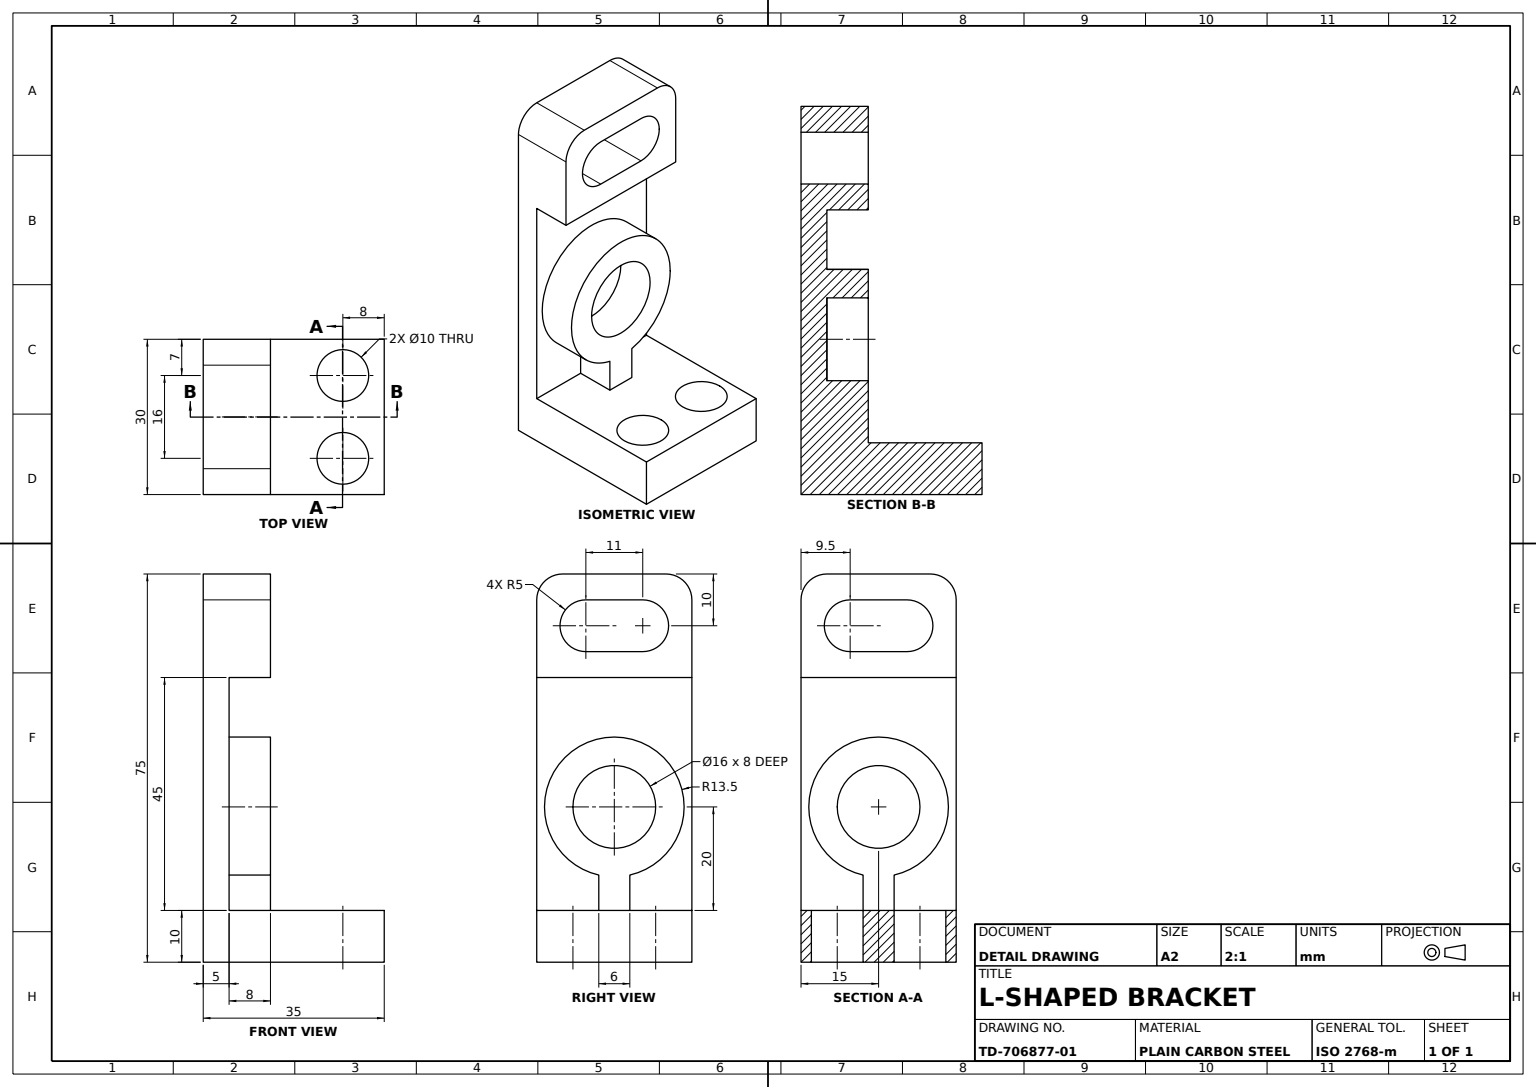
from build123d import *

# Parameters (mm, degrees)
BASE_PLATE_SKETCH_W     = 35
BASE_PLATE_SKETCH_H     = 10
BASE_PLATE_DEPTH        = 30
UPRIGHT_WALL_SKETCH_W   = 5
UPRIGHT_WALL_SKETCH_H   = 45
UPRIGHT_WALL_DEPTH      = 30
MOUNTING_HOLES_SKETCH_R = 5
MOUNTING_HOLES_2X_DEPTH = 30
TOP_LUG_DEPTH           = 8
TOP_LUG_DEPTH_BACK      = 5
LUG_SLOT_DEPTH          = 84.719770664
RING_BOSS_SKETCH_R      = 8
RING_BOSS_DEPTH         = 8


with BuildPart() as part:
    # Base Plate Sketch → Base Plate (new body)
    with BuildSketch(Plane.XY):
        with Locations((17.5, 5)):
            Rectangle(BASE_PLATE_SKETCH_W, BASE_PLATE_SKETCH_H)
    extrude(amount=-BASE_PLATE_DEPTH)

    # Upright Wall Sketch → Upright Wall (add)
    with BuildSketch(Plane.XY):
        with Locations((2.5, 32.5)):
            Rectangle(UPRIGHT_WALL_SKETCH_W, UPRIGHT_WALL_SKETCH_H)
    extrude(amount=-UPRIGHT_WALL_DEPTH)

    # Mounting Holes Sketch → Mounting Holes 2x (cut)
    with BuildSketch(Plane(origin=(0, 10, 0), x_dir=(1, 0, 0), z_dir=(0, 1, 0))):
        with Locations(Location((27, 23, 0), (0, 0, 270))):
            Circle(MOUNTING_HOLES_SKETCH_R)
        with Locations(Location((27, 7, 0), (0, 0, 270))):
            Circle(MOUNTING_HOLES_SKETCH_R)
    extrude(amount=-MOUNTING_HOLES_2X_DEPTH, mode=Mode.SUBTRACT)

    # Top Lug Sketch → Top Lug (add, two sides: drawn at the far end of the back side and taken through both)
    with BuildSketch(Plane(origin=(5, 0, 0), x_dir=(0, 0, -1), z_dir=(1, 0, 0)).offset(-TOP_LUG_DEPTH_BACK)):
        with BuildLine():
            Line((0, 55), (30, 55))
            Line((30, 55), (30, 70))
            ThreePointArc((30, 70), (28.535533906, 73.535533906), (25, 75))
            Line((25, 75), (5, 75))
            ThreePointArc((5, 75), (1.464466094, 73.535533906), (0, 70))
            Line((0, 70), (0, 55))
        make_face()
    extrude(amount=TOP_LUG_DEPTH + TOP_LUG_DEPTH_BACK)

    # Lug Slot Sketch → Lug Slot (cut, through all)
    with BuildSketch(Plane(origin=(13, 0, 0), x_dir=(0, 0, -1), z_dir=(1, 0, 0))):
        with BuildLine():
            Line((9.5, 70), (20.5, 70))
            ThreePointArc((20.5, 70), (25.5, 65), (20.5, 60))
            Line((20.5, 60), (9.5, 60))
            ThreePointArc((9.5, 60), (4.5, 65), (9.5, 70))
        make_face()
    extrude(amount=-LUG_SLOT_DEPTH, mode=Mode.SUBTRACT)

    # Ring Boss Sketch → Ring Boss (add)
    with BuildSketch(Plane(origin=(5, 0, 0), x_dir=(0, 0, -1), z_dir=(1, 0, 0))):
        with BuildLine():
            Line((12, 16.837553419), (12, 10))
            Line((12, 10), (18, 10))
            Line((18, 10), (18, 16.837553419))
            ThreePointArc((18, 16.837553419), (15, 43.5), (12, 16.837553419))
        make_face()
        with Locations((15, 30)):
            Circle(RING_BOSS_SKETCH_R, mode=Mode.SUBTRACT)
    extrude(amount=RING_BOSS_DEPTH)


solid = part.part
